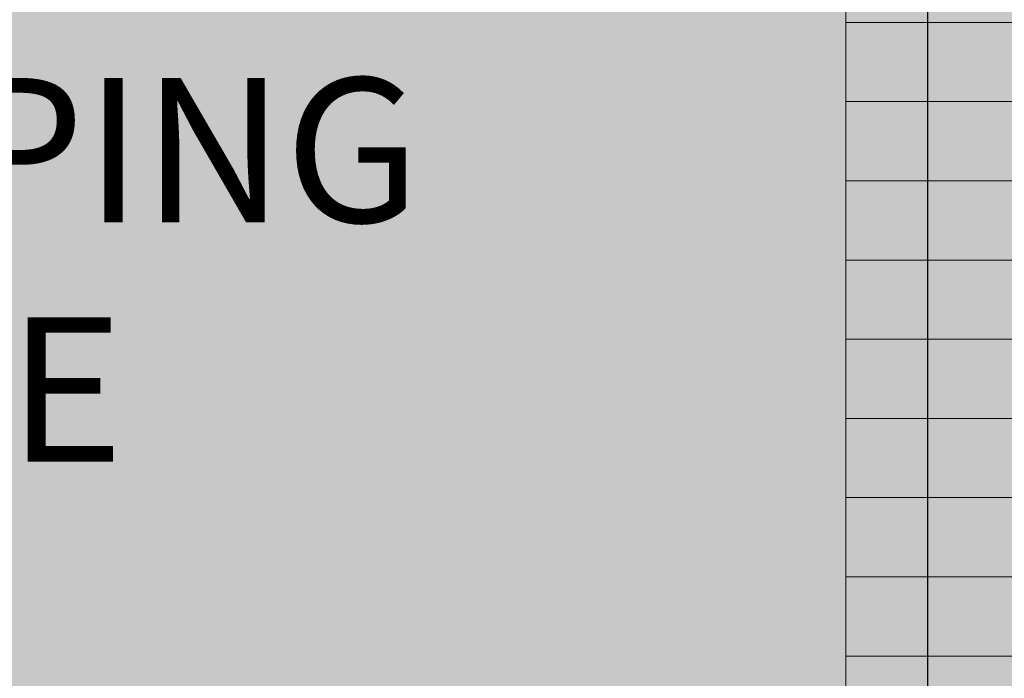
# Model space of a CAD drawing. Units: inches. Extents: x 1704 to 6393, y -157 to 1172.
# Tile 74 of 122: x 1987 to 2081, y 920 to 983. Entities that reach past the tile are written whole.
import ezdxf

# ---------------------------------------------------------------- set-up
doc = ezdxf.new("R2010")
doc.units = ezdxf.units.IN
doc.header["$MEASUREMENT"] = 0
for name, color, linetype, lineweight in [('A-ANNO-DIMS', 7, 'Continuous', 13), ('A-AREA-IDEN', 7, 'Continuous', 18), ('L-DECK-PLNK-PATT', 250, 'Continuous', 13), ('L-HRDS', 8, 'Continuous', 18)]:
    doc.layers.add(name, color=color, linetype=linetype, lineweight=lineweight)
doc.layers.add('L-DECK-PATT', color=35, linetype='Continuous', lineweight=13, true_color=0xa6725b)
doc.layers.add('L-HRDS-PATT', color=9, linetype='Continuous', lineweight=13, true_color=0xc5c1ba)
doc.styles.get("Standard").update_dxf_attribs({"font": 'arial.ttf'})
doc.dimstyles.get("Standard").update_dxf_attribs({"dimtxt": 6, "dimasz": 2, "dimexe": 0.18, "dimexo": 0.0625, "dimgap": 0.09, "dimtad": 0, "dimtih": 1, "dimtoh": 1, "dimdec": 1, "dimzin": 0, "dimdsep": 46, "dimlunit": 3, "dimtxsty": 'Standard', "dimblk": 'ARCHTICK', "dimcen": 0.09, "dimadec": 0, "dimazin": 0, "dimtfac": 1, "dimtdec": 1, "dimtofl": 0, "dimtmove": 0, "dimatfit": 3, "dimfxl": 1, "dimtolj": 1, "dimtzin": 0, "dimarcsym": 0})

# ---------------------------------------------------------------- blocks, each defined once
blk = doc.blocks.new('_ArchTick')
at = {"color": 0, "linetype": 'ByBlock', "const_width": 0.15}
blk.add_lwpolyline([(-0.5, -0.5), (0.5, 0.5)], dxfattribs=at)
blk = doc.blocks.new('*D92')
at = {"layer": 'A-ANNO-DIMS', "color": 0, "lineweight": -2, "transparency": 16777216}
for p, q in [((2073.349, 895.275), (2073.349, 1105.287)), ((2073.349, 1105.107), (2332.661, 1105.107)), ((2605.349, 1105.107), (2346.036, 1105.107)), ((2605.349, 895.275), (2605.349, 1105.287))]:
    blk.add_line(p, q, dxfattribs=at)
at = {"layer": 'Defpoints', "color": 0, "lineweight": -3, "transparency": 16777216}
for p in [(2605.349, 1105.107), (2073.349, 895.213), (2605.349, 895.213)]:
    blk.add_point(p, dxfattribs=at)
at = {"layer": 'A-ANNO-DIMS', "color": 0, "lineweight": -2, "transparency": 16777216, "xscale": 2, "yscale": 2, "zscale": 2, "rotation": 180}
blk.add_blockref('_ArchTick', (2073.349, 1105.107), dxfattribs=at)
at = {"layer": 'A-ANNO-DIMS', "color": 0, "lineweight": -2, "transparency": 16777216, "xscale": 2, "yscale": 2, "zscale": 2}
blk.add_blockref('_ArchTick', (2605.349, 1105.107), dxfattribs=at)
at = {"layer": 'A-ANNO-DIMS', "color": 0, "transparency": 16777216, "insert": (2339.349, 1105.107), "char_height": 6, "attachment_point": 5}
blk.add_mtext('\\A1;532', dxfattribs=at)
blk = doc.blocks.new('*D94')
at = {"layer": 'A-ANNO-DIMS', "color": 0, "lineweight": -2, "transparency": 16777216}
for p, q in [((1898.349, 895.275), (1898.349, 1105.287)), ((1898.349, 1105.107), (1979.39, 1105.107)), ((2073.349, 1105.107), (1992.307, 1105.107)), ((2073.349, 895.275), (2073.349, 1105.287))]:
    blk.add_line(p, q, dxfattribs=at)
at = {"layer": 'Defpoints', "color": 0, "lineweight": -3, "transparency": 16777216}
for p in [(2073.349, 1105.107), (1898.349, 895.213), (2073.349, 895.213)]:
    blk.add_point(p, dxfattribs=at)
at = {"layer": 'A-ANNO-DIMS', "color": 0, "lineweight": -2, "transparency": 16777216, "xscale": 2, "yscale": 2, "zscale": 2, "rotation": 180}
blk.add_blockref('_ArchTick', (1898.349, 1105.107), dxfattribs=at)
at = {"layer": 'A-ANNO-DIMS', "color": 0, "lineweight": -2, "transparency": 16777216, "xscale": 2, "yscale": 2, "zscale": 2}
blk.add_blockref('_ArchTick', (2073.349, 1105.107), dxfattribs=at)
at = {"layer": 'A-ANNO-DIMS', "color": 0, "transparency": 16777216, "insert": (1985.849, 1105.107), "char_height": 6, "attachment_point": 5}
blk.add_mtext('\\A1;175', dxfattribs=at)

msp = doc.modelspace()

# ---------------------------------------------------------------- hatches: boundary and pattern name
at = {"layer": 'L-DECK-PATT', "transparency": 33554544}
h = msp.add_hatch(color=256, dxfattribs=at)
h.dxf.hatch_style = 1
h.paths.add_polyline_path([(2329.589, 1033.213), (2065.589, 1033.213), (2065.589, 895.213), (2167.349, 895.213), (2263.349, 895.213), (2263.349, 903.213), (2273.349, 903.213), (2273.349, 895.213), (2329.589, 895.213)])
h.paths.add_polyline_path([(2664.349, 1033.213), (2333.589, 1033.213), (2333.589, 895.213), (2465.349, 895.213), (2469.181, 895.213), (2470.482, 895.213), (2508.215, 895.213), (2509.516, 895.213), (2513.349, 895.213), (2533.349, 895.213), (2581.349, 895.213), (2605.349, 895.213), (2664.349, 895.213)])
h.paths.add_polyline_path([(2333.589, 1033.213), (2329.589, 1033.213), (2329.589, 895.213), (2333.589, 895.213)])
at = {"layer": 'L-DECK-PLNK-PATT'}
h = msp.add_hatch(dxfattribs=at)
h.set_pattern_fill('LINE', color=256, scale=60)
h.paths.add_polyline_path([(2329.589, 1033.213), (2065.589, 1033.213), (2065.589, 895.213), (2167.349, 895.213), (2263.349, 895.213), (2263.349, 903.213), (2273.349, 903.213), (2273.349, 895.213), (2329.589, 895.213)])
h.paths.add_polyline_path([(2664.349, 1033.213), (2333.589, 1033.213), (2333.589, 895.213), (2465.349, 895.213), (2469.181, 895.213), (2470.482, 895.213), (2508.215, 895.213), (2509.516, 895.213), (2513.349, 895.213), (2533.349, 895.213), (2581.349, 895.213), (2605.349, 895.213), (2664.349, 895.213)])
h.paths.add_polyline_path([(2333.589, 1033.213), (2329.589, 1033.213), (2329.589, 895.213), (2333.589, 895.213)])
at = {"layer": 'L-HRDS-PATT', "transparency": 33554643}
h = msp.add_hatch(color=256, dxfattribs=at)
h.dxf.hatch_style = 1
h.paths.add_polyline_path([(2065.589, 1033.213), (1898.349, 1033.213), (1898.349, 895.213), (2065.589, 895.213)])

# ---------------------------------------------------------------- linework, layer by layer
at = {"layer": 'L-HRDS'}
msp.add_line((2065.589, 895.213), (2065.589, 1033.213), dxfattribs=at)

# ---------------------------------------------------------------- texts
at = {"layer": 'A-AREA-IDEN'}
for s, p in [('STEPPING', (1936.64, 963.579)), ('STONE', (1936.64, 940.915))]:
    msp.add_text(s, height=13.6672, dxfattribs=at).set_placement(p)

# ---------------------------------------------------------------- dimensions: what is measured, and where the dimension line sits
at = {"layer": 'A-ANNO-DIMS'}
for base, p1, p2, picture, middle in [((2073.349, 1105.107), (1898.349, 895.213), (2073.349, 895.213), '*D94', (1985.849, 1105.107)), ((2605.349, 1105.107), (2073.349, 895.213), (2605.349, 895.213), '*D92', (2339.349, 1105.107))]:
    dim = msp.add_linear_dim(base=base, p1=p1, p2=p2, dimstyle='Standard', override={"dimdec": 0, "dimlfac": 1, "dimrnd": 0, "dimzin": 0, "dimdsep": 46, "dimlunit": 2}, dxfattribs=at)
    dim.commit()
    dim.dimension.update_dxf_attribs({"geometry": picture, "text_midpoint": middle})

doc.saveas('drawing.dxf')
